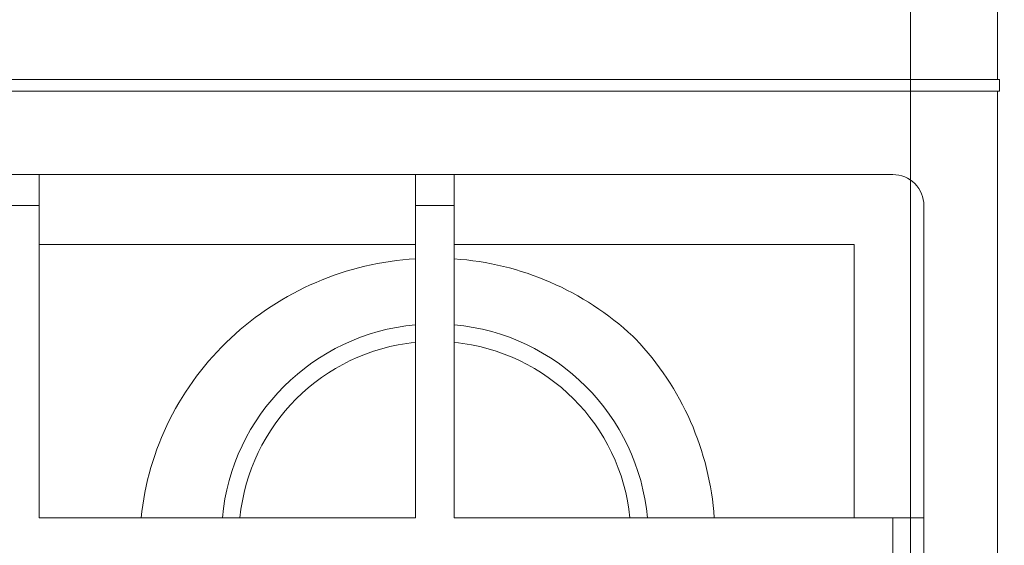
# Model space of a CAD drawing. Units: inches. Extents: x -1198 to -69, y -512 to 437.
# Tile 9 of 50: x -956.36 to -945.11, y 176.14 to 182.14. Entities that reach past the tile are written whole.
import ezdxf

# ---------------------------------------------------------------- set-up
doc = ezdxf.new("R2010")
doc.units = ezdxf.units.IN
doc.header["$MEASUREMENT"] = 0
for name, color, linetype, lineweight in [('0_Pen_No__7', 7, 'Continuous', 18), ('A-ANNO-DIMS', 2, 'Continuous', 18), ('A-EQPM', 60, 'Continuous', 18)]:
    doc.layers.add(name, color=color, linetype=linetype, lineweight=lineweight)
doc.styles.get("Standard").update_dxf_attribs({"font": 'arial.ttf'})
doc.dimstyles.get("Standard").update_dxf_attribs({"dimtxt": 6, "dimasz": 6, "dimexe": 0.18, "dimexo": 0.0625, "dimgap": 0.09, "dimtad": 0, "dimtih": 1, "dimtoh": 1, "dimdec": 0, "dimzin": 0, "dimdsep": 46, "dimlunit": 4, "dimtxsty": 'Standard', "dimblk": 'OBLIQUE', "dimcen": 0.09, "dimadec": 0, "dimazin": 0, "dimtfac": 1, "dimtdec": 0, "dimtofl": 0, "dimtmove": 0, "dimatfit": 3, "dimfxl": 1, "dimtolj": 1, "dimtzin": 0, "dimarcsym": 0})

# ---------------------------------------------------------------- blocks, each defined once
blk = doc.blocks.new('new block')
at = {"layer": '0_Pen_No__7'}
for p, q in [((-328.59, 234.26), (-328.59, 223)), ((-190.06, 143.6), (-80.82, 143.6)), ((-201.32, 132.33), (-190.06, 132.33)), ((-80.82, 132.33), (-69.55, 132.33)), ((-359, 99.11), (485.68, 99.11)), ((485.68, 95.73), (-359, 95.73))]:
    blk.add_line(p, q, dxfattribs=at)
for points in [[(-354.49, 596.91), (481.18, 596.91, -0.414214), (485.68, 592.4), (485.68, 99.11), (486.24, 99.11), (486.24, 95.73), (485.68, 95.73), (485.68, 4.5, -0.414214), (481.18, 0), (-354.49, 0, -0.414214), (-359, 4.5), (-359, 95.73), (-359.56, 95.73), (-359.56, 99.11), (-359, 99.11), (-359, 592.4, -0.414214)], [(464.28, 132.33), (464.28, 567.06, 0.414214), (455.27, 576.07), (-328.59, 576.07, 0.414214), (-337.6, 567.06), (-337.6, 132.33, 0.414214), (-328.59, 123.32), (455.27, 123.32, 0.414214)]]:
    blk.add_lwpolyline(points, format="xyb", close=True, dxfattribs=at)
blk.add_lwpolyline([(-333.7, 12.95), (460.3, 12.95), (460.3, 570.44), (-333.7, 570.44)], close=True, dxfattribs=at)
for points in [[(-201.32, 123.32), (-201.32, 223), (-337.6, 223)], [(-317.33, 223), (-317.33, 143.6), (-201.32, 143.6)], [(-80.82, 123.32), (-80.82, 223), (-190.06, 223), (-190.06, 123.32)], [(-190.06, 147.76), (-188.21, 147.89), (-186.35, 148.06), (-184.5, 148.28), (-182.66, 148.53), (-180.82, 148.83), (-178.99, 149.16), (-177.16, 149.53), (-175.35, 149.94), (-173.54, 150.39), (-171.74, 150.88), (-169.96, 151.41), (-168.18, 151.98), (-166.42, 152.58), (-164.68, 153.23), (-162.94, 153.9), (-161.22, 154.62), (-159.52, 155.37), (-157.84, 156.16), (-156.17, 156.99), (-154.52, 157.85), (-152.89, 158.75), (-151.28, 159.68), (-149.69, 160.65), (-148.12, 161.65), (-146.57, 162.68), (-145.04, 163.75), (-143.54, 164.85), (-142.07, 165.98), (-140.61, 167.15), (-139.19, 168.34), (-137.79, 169.57), (-136.42, 170.82), (-135.07, 172.11), (-133.75, 173.43), (-132.47, 174.77), (-131.21, 176.14), (-129.98, 177.54), (-128.79, 178.97), (-127.62, 180.42), (-126.49, 181.9), (-125.39, 183.4), (-124.33, 184.93), (-123.3, 186.48), (-122.3, 188.05), (-121.34, 189.64), (-120.42, 191.26), (-119.53, 192.89), (-118.68, 194.55), (-117.87, 196.22), (-117.09, 197.91), (-116.36, 199.62), (-115.66, 201.35), (-115, 203.09), (-114.38, 204.84), (-113.8, 206.61), (-113.26, 208.39), (-112.76, 210.19), (-112.31, 211.99), (-111.89, 213.81), (-111.52, 215.63), (-111.19, 217.46), (-110.9, 219.3), (-110.65, 221.15), (-110.45, 222.99)]]:
    blk.add_lwpolyline(points, dxfattribs=at)
for centre, radius, start, end in [((-193.43, 228.67), 83.53, 183.8969, 223.6071), ((-195.69, 228.63), 61.94, 185.2164, 264.7832), ((-195.69, 228.63), 56.88, 185.6822, 264.3178), ((-195.69, 228.63), 61.94, 275.2168, 354.7836), ((-195.69, 228.63), 56.88, 275.6822, 354.3178), ((-239.43, 184.87), 20.01, 223.6326, 226.8635), ((-195.64, 231.83), 84.22, 226.9693, 266.1293)]:
    blk.add_arc(centre, radius, start, end, dxfattribs=at)
blk = doc.blocks.new('_Oblique')
at = {"color": 0, "linetype": 'ByBlock', "lineweight": -2}
blk.add_line((-0.5, -0.5), (0.5, 0.5), dxfattribs=at)
blk = doc.blocks.new('*D50')
at = {"layer": 'A-ANNO-DIMS', "color": 0, "lineweight": -2, "ltscale": 10, "transparency": 16777216}
for p, q in [((-978.462, 185.29), (-978.462, 190.403)), ((-945.163, 185.29), (-945.163, 190.403)), ((-978.462, 190.223), (-984.462, 190.223)), ((-945.163, 190.223), (-978.462, 190.223))]:
    blk.add_line(p, q, dxfattribs=at)
at = {"layer": 'DEFPOINTS', "color": 0, "ltscale": 10, "transparency": 16777216}
for p in [(-978.462, 190.223), (-978.462, 185.228), (-945.163, 185.228)]:
    blk.add_point(p, dxfattribs=at)
at = {"layer": 'A-ANNO-DIMS', "color": 0, "lineweight": -2, "ltscale": 10, "transparency": 16777216, "xscale": 6, "yscale": 6, "zscale": 6, "rotation": 180}
blk.add_blockref('_Oblique', (-978.462, 190.223), dxfattribs=at)
at = {"layer": 'A-ANNO-DIMS', "color": 0, "lineweight": -2, "ltscale": 10, "transparency": 16777216, "xscale": 6, "yscale": 6, "zscale": 6}
blk.add_blockref('_Oblique', (-945.163, 190.223), dxfattribs=at)
at = {"layer": 'A-ANNO-DIMS', "color": 0, "ltscale": 10, "transparency": 16777216, "insert": (-1009.24, 190.223), "char_height": 6, "attachment_point": 5}
blk.add_mtext('\\A1;HOB 33 TYP.', dxfattribs=at)

msp = doc.modelspace()

# ---------------------------------------------------------------- block references
at = {"layer": 'A-EQPM', "xscale": 0.0393700787401575, "yscale": 0.0393700787401575, "zscale": 0.0393700787401575, "rotation": 180}
msp.add_blockref('new block', (-959.3186, 185.2277), dxfattribs=at)

# ---------------------------------------------------------------- dimensions: what is measured, and where the dimension line sits
at = {"layer": 'A-ANNO-DIMS', "ltscale": 10}
dim = msp.add_linear_dim(base=(-978.4621, 190.2226), p1=(-945.1627, 185.2277), p2=(-978.4621, 185.2277), angle=180, text='HOB <> TYP.', dimstyle='Standard', override={"dimdec": 0, "dimlfac": 1, "dimrnd": 0, "dimzin": 0, "dimdsep": 46, "dimlunit": 2}, dxfattribs=at)
dim.commit()
dim.dimension.update_dxf_attribs({"geometry": '*D50', "text_midpoint": (-1009.2397, 190.2226)})

doc.saveas('drawing.dxf')
